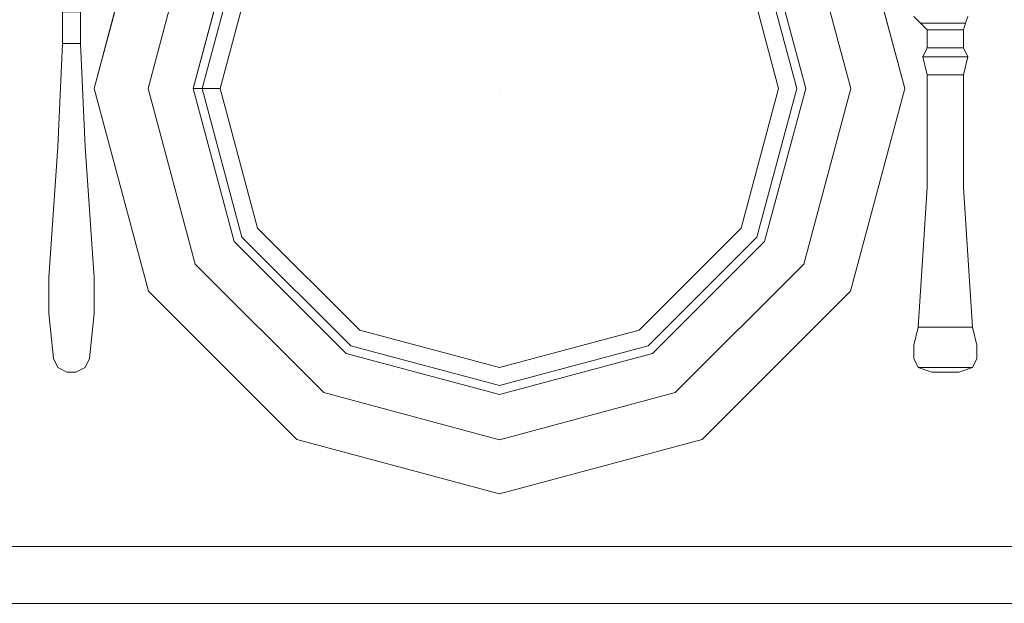
# Model space of a CAD drawing. Units: inches. Extents: x 375 to 1122, y 27 to 1069.
# Tile 10 of 155: x 719.12 to 732.58, y 254.7 to 262.68. Entities that reach past the tile are written whole.
import ezdxf

# ---------------------------------------------------------------- set-up
doc = ezdxf.new("R2010")
doc.units = ezdxf.units.IN
doc.layers.add('Furniture', color=30, linetype='Continuous', lineweight=18)

# ---------------------------------------------------------------- blocks, each defined once
blk = doc.blocks.new('A$C403C54AD')
for p, q in [((2.27071, 1.26108, -0.0006), (2.27071, 0.79569, -0.0006)), ((2.2901, 1.26108, -0.0006), (2.2901, 0.79569, -0.0006))]:
    blk.add_line(p, q)
for points, invisible_edges in [([(2.19569, 1.17996, -0.05014), (2.19569, 1.16149, -0.05014), (2.20185, 1.15995, -0.0486), (2.20185, 1.1815, -0.0486)], 4), ([(2.19569, 1.17996, -0.05938), (2.19569, 1.16149, -0.05938), (2.20185, 1.15995, -0.06091), (2.20185, 1.1815, -0.06091)], 4), ([(2.20185, 1.15995, -0.0486), (2.20185, 1.1815, -0.0486), (2.20647, 1.1815, -0.05014), (2.20647, 1.15995, -0.05014)], 5), ([(2.20185, 1.15995, -0.06091), (2.20185, 1.1815, -0.06091), (2.20647, 1.1815, -0.05938), (2.20647, 1.15995, -0.05938)], 5), ([(2.20647, 1.1815, -0.05014), (2.20647, 1.15995, -0.05014), (2.20954, 1.16149, -0.05168), (2.20954, 1.17996, -0.05168)], 1), ([(2.20647, 1.1815, -0.05938), (2.20647, 1.15995, -0.05938), (2.20954, 1.16149, -0.05784), (2.20954, 1.17996, -0.05784)], 1), ([(2.08949, 1.15995, -0.05399), (2.08949, 1.17842, -0.05399), (2.0918, 1.17765, -0.05322), (2.0918, 1.16226, -0.05322)], 1), ([(2.08949, 1.15995, -0.05553), (2.08949, 1.17842, -0.05553), (2.0918, 1.17765, -0.0563), (2.0918, 1.16226, -0.0563)], 1), ([(2.0918, 1.17765, -0.0563), (2.0918, 1.17765, -0.05322), (2.08949, 1.17842, -0.05399), (2.08949, 1.17842, -0.05553)], 5), ([(2.0941, 1.17688, -0.05014), (2.0941, 1.17688, -0.05938), (2.0918, 1.17765, -0.0563), (2.0918, 1.17765, -0.05322)], 5), ([(2.14798, 1.17688, -0.0486), (2.14798, 1.16457, -0.0486), (2.17106, 1.16303, -0.0486), (2.17106, 1.17842, -0.0486)], 5), ([(2.14798, 1.17688, -0.06091), (2.14798, 1.16457, -0.06091), (2.17106, 1.16303, -0.06091), (2.17106, 1.17842, -0.06091)], 5), ([(2.17106, 1.16303, -0.0486), (2.17106, 1.17842, -0.0486), (2.19569, 1.17996, -0.05014), (2.19569, 1.16149, -0.05014)], 1), ([(2.17106, 1.16303, -0.06091), (2.17106, 1.17842, -0.06091), (2.19569, 1.17996, -0.05938), (2.19569, 1.16149, -0.05938)], 1), ([(2.10026, 1.17688, -0.05938), (2.10026, 1.17688, -0.05014), (2.0941, 1.17688, -0.05014), (2.0941, 1.17688, -0.05938)], 4), ([(2.1095, 1.16457, -0.05014), (2.1095, 1.17688, -0.05014), (2.14798, 1.17688, -0.0486), (2.14798, 1.16457, -0.0486)], 4), ([(2.1095, 1.16457, -0.05938), (2.1095, 1.17688, -0.05938), (2.14798, 1.17688, -0.06091), (2.14798, 1.16457, -0.06091)], 4), ([(2.0918, 1.16226, -0.05322), (2.0918, 1.16226, -0.0563), (2.0941, 1.16457, -0.05938), (2.0941, 1.16457, -0.05014)], 5), ([(2.0941, 1.16457, -0.05938), (2.0941, 1.16457, -0.05014), (2.10026, 1.16457, -0.05014), (2.10026, 1.16457, -0.05938)], 1), ([(2.08949, 1.15995, -0.05553), (2.08949, 1.15995, -0.05399), (2.0918, 1.16226, -0.05322), (2.0918, 1.16226, -0.0563)], 5), ([(2.17876, 0.86443, -0.04825), (2.17876, 0.87982, -0.04825), (2.13412, 0.87674, -0.04587), (2.13412, 0.8675, -0.04587)], 5), ([(2.17876, 0.86443, -0.05289), (2.17876, 0.87982, -0.05289), (2.13412, 0.87674, -0.04895), (2.13412, 0.8675, -0.04895)], 5), ([(2.17876, 0.87982, -0.05289), (2.17876, 0.87982, -0.04825), (2.13412, 0.87674, -0.04587), (2.13412, 0.87674, -0.04895)], 4), ([(2.19107, 0.87982, -0.04858), (2.19107, 0.86443, -0.04858), (2.17876, 0.86443, -0.04825), (2.17876, 0.87982, -0.04825)], 5), ([(2.19107, 0.87982, -0.05321), (2.19107, 0.86443, -0.05321), (2.17876, 0.86443, -0.05289), (2.17876, 0.87982, -0.05289)], 5), ([(2.20647, 0.86596, -0.04855), (2.20647, 0.87828, -0.04855), (2.19107, 0.87982, -0.04858), (2.19107, 0.86443, -0.04858)], 5), ([(2.20647, 0.86596, -0.05318), (2.20647, 0.87828, -0.05318), (2.19107, 0.87982, -0.05321), (2.19107, 0.86443, -0.05321)], 5), ([(2.20954, 0.87674, -0.0483), (2.20954, 0.8675, -0.0483), (2.20647, 0.86596, -0.04855), (2.20647, 0.87828, -0.04855)], 5), ([(2.20954, 0.87674, -0.05294), (2.20954, 0.8675, -0.05294), (2.20647, 0.86596, -0.05318), (2.20647, 0.87828, -0.05318)], 5), ([(2.09872, 0.8752, -0.04555), (2.09872, 0.8752, -0.04296), (2.08795, 0.8752, -0.04504), (2.08795, 0.8752, -0.04763)], 5), ([(2.13412, 0.87674, -0.04587), (2.13412, 0.8675, -0.04587), (2.09872, 0.86904, -0.04296), (2.09872, 0.8752, -0.04296)], 1), ([(2.13412, 0.87674, -0.04587), (2.13412, 0.87674, -0.04895), (2.09872, 0.8752, -0.04555), (2.09872, 0.8752, -0.04296)], 5), ([(2.13412, 0.87674, -0.04895), (2.13412, 0.8675, -0.04895), (2.09872, 0.86904, -0.04555), (2.09872, 0.8752, -0.04555)], 1), ([(2.21108, 0.87058, -0.04847), (2.21108, 0.87366, -0.04847), (2.20954, 0.87674, -0.0483), (2.20954, 0.8675, -0.0483)], 4), ([(2.21108, 0.87058, -0.0526), (2.21108, 0.87366, -0.0526), (2.20954, 0.87674, -0.05294), (2.20954, 0.8675, -0.05294)], 4), ([(2.08795, 0.86904, -0.04763), (2.08795, 0.86904, -0.04504), (2.09872, 0.86904, -0.04296), (2.09872, 0.86904, -0.04555)], 5), ([(2.09872, 0.86904, -0.04296), (2.09872, 0.86904, -0.04555), (2.13412, 0.8675, -0.04895), (2.13412, 0.8675, -0.04587)], 5), ([(2.13412, 0.8675, -0.04895), (2.13412, 0.8675, -0.04587), (2.17876, 0.86443, -0.04825), (2.17876, 0.86443, -0.05289)], 1)]:
    blk.add_3dface(points, dxfattribs=dict(invisible_edges=invisible_edges))
for points in [[(2.20185, 1.1815, -0.06091), (2.20185, 1.1815, -0.0486), (2.19569, 1.17996, -0.05014), (2.19569, 1.17996, -0.05938)], [(2.20647, 1.1815, -0.05014), (2.20647, 1.1815, -0.05938), (2.20185, 1.1815, -0.06091), (2.20185, 1.1815, -0.0486)], [(2.20954, 1.17996, -0.05168), (2.20954, 1.17996, -0.05784), (2.20647, 1.1815, -0.05938), (2.20647, 1.1815, -0.05014)], [(2.0918, 1.16226, -0.05322), (2.0918, 1.17765, -0.05322), (2.0941, 1.17688, -0.05014), (2.0941, 1.16457, -0.05014)], [(2.0918, 1.16226, -0.0563), (2.0918, 1.17765, -0.0563), (2.0941, 1.17688, -0.05938), (2.0941, 1.16457, -0.05938)], [(2.10026, 1.16457, -0.05014), (2.10026, 1.17688, -0.05014), (2.10334, 1.17842, -0.0486), (2.10334, 1.16303, -0.0486)], [(2.10026, 1.16457, -0.05938), (2.10026, 1.17688, -0.05938), (2.10334, 1.17842, -0.06091), (2.10334, 1.16303, -0.06091)], [(2.10334, 1.17842, -0.0486), (2.10334, 1.17842, -0.06091), (2.10026, 1.17688, -0.05938), (2.10026, 1.17688, -0.05014)], [(2.10334, 1.17842, -0.0486), (2.10334, 1.16303, -0.0486), (2.1095, 1.16457, -0.05014), (2.1095, 1.17688, -0.05014)], [(2.10334, 1.17842, -0.06091), (2.10334, 1.16303, -0.06091), (2.1095, 1.16457, -0.05938), (2.1095, 1.17688, -0.05938)], [(2.1095, 1.17688, -0.05938), (2.1095, 1.17688, -0.05014), (2.10334, 1.17842, -0.0486), (2.10334, 1.17842, -0.06091)], [(2.17106, 1.17842, -0.06091), (2.17106, 1.17842, -0.0486), (2.14798, 1.17688, -0.0486), (2.14798, 1.17688, -0.06091)], [(2.19569, 1.17996, -0.05014), (2.19569, 1.17996, -0.05938), (2.17106, 1.17842, -0.06091), (2.17106, 1.17842, -0.0486)], [(2.20954, 1.16149, -0.05168), (2.20954, 1.17996, -0.05168), (2.21108, 1.17534, -0.05476), (2.21108, 1.16611, -0.05476)], [(2.21108, 1.17534, -0.05476), (2.21108, 1.17534, -0.05476), (2.20954, 1.17996, -0.05168), (2.20954, 1.17996, -0.05784)], [(2.20954, 1.16149, -0.05784), (2.20954, 1.17996, -0.05784), (2.21108, 1.17534, -0.05476), (2.21108, 1.16611, -0.05476)], [(2.0941, 1.17688, -0.05014), (2.0941, 1.16457, -0.05014), (2.10026, 1.16457, -0.05014), (2.10026, 1.17688, -0.05014)], [(2.0941, 1.17688, -0.05938), (2.0941, 1.16457, -0.05938), (2.10026, 1.16457, -0.05938), (2.10026, 1.17688, -0.05938)], [(2.14798, 1.17688, -0.0486), (2.14798, 1.17688, -0.06091), (2.1095, 1.17688, -0.05938), (2.1095, 1.17688, -0.05014)], [(2.10026, 1.16457, -0.05014), (2.10026, 1.16457, -0.05938), (2.10334, 1.16303, -0.06091), (2.10334, 1.16303, -0.0486)], [(2.10334, 1.16303, -0.06091), (2.10334, 1.16303, -0.0486), (2.1095, 1.16457, -0.05014), (2.1095, 1.16457, -0.05938)], [(2.1095, 1.16457, -0.05014), (2.1095, 1.16457, -0.05938), (2.14798, 1.16457, -0.06091), (2.14798, 1.16457, -0.0486)], [(2.14798, 1.16457, -0.06091), (2.14798, 1.16457, -0.0486), (2.17106, 1.16303, -0.0486), (2.17106, 1.16303, -0.06091)], [(2.20954, 1.16149, -0.05168), (2.20954, 1.16149, -0.05784), (2.21108, 1.16611, -0.05476)], [(2.17106, 1.16303, -0.0486), (2.17106, 1.16303, -0.06091), (2.19569, 1.16149, -0.05938), (2.19569, 1.16149, -0.05014)], [(2.19569, 1.16149, -0.05938), (2.19569, 1.16149, -0.05014), (2.20185, 1.15995, -0.0486), (2.20185, 1.15995, -0.06091)], [(2.20647, 1.15995, -0.05938), (2.20647, 1.15995, -0.05014), (2.20954, 1.16149, -0.05168), (2.20954, 1.16149, -0.05784)], [(2.20185, 1.15995, -0.0486), (2.20185, 1.15995, -0.06091), (2.20647, 1.15995, -0.05938), (2.20647, 1.15995, -0.05014)], [(2.19107, 0.87982, -0.04858), (2.19107, 0.87982, -0.05321), (2.17876, 0.87982, -0.05289), (2.17876, 0.87982, -0.04825)], [(2.20647, 0.87828, -0.05318), (2.20647, 0.87828, -0.04855), (2.19107, 0.87982, -0.04858), (2.19107, 0.87982, -0.05321)], [(2.20954, 0.87674, -0.0483), (2.20954, 0.87674, -0.05294), (2.20647, 0.87828, -0.05318), (2.20647, 0.87828, -0.04855)], [(2.09872, 0.86904, -0.04296), (2.09872, 0.8752, -0.04296), (2.08795, 0.8752, -0.04504), (2.08795, 0.86904, -0.04504)], [(2.09872, 0.86904, -0.04555), (2.09872, 0.8752, -0.04555), (2.08795, 0.8752, -0.04763), (2.08795, 0.86904, -0.04763)], [(2.21108, 0.87366, -0.0526), (2.21108, 0.87366, -0.04847), (2.20954, 0.87674, -0.0483), (2.20954, 0.87674, -0.05294)], [(2.21108, 0.87058, -0.04847), (2.21108, 0.87058, -0.0526), (2.21108, 0.87366, -0.0526), (2.21108, 0.87366, -0.04847)], [(2.20954, 0.8675, -0.05294), (2.20954, 0.8675, -0.0483), (2.21108, 0.87058, -0.04847), (2.21108, 0.87058, -0.0526)], [(2.19107, 0.86443, -0.05321), (2.19107, 0.86443, -0.04858), (2.20647, 0.86596, -0.04855), (2.20647, 0.86596, -0.05318)], [(2.20647, 0.86596, -0.04855), (2.20647, 0.86596, -0.05318), (2.20954, 0.8675, -0.05294), (2.20954, 0.8675, -0.0483)], [(2.17876, 0.86443, -0.04825), (2.17876, 0.86443, -0.05289), (2.19107, 0.86443, -0.05321), (2.19107, 0.86443, -0.04858)]]:
    blk.add_3dface(points)
at = {"linetype": 'ByBlock'}
for points, invisible_edges in [([(2.11411, 1.15687, -0.03783), (2.11411, 1.1384, -0.03783), (2.05409, 1.12232, -0.03783), (2.04485, 1.13831, -0.03783)], 5), ([(2.11411, 1.12301, -0.05168), (2.11411, 1.15687, -0.04244), (2.04485, 1.13831, -0.04244), (2.06178, 1.10899, -0.05168)], 5), ([(2.18338, 1.13831, -0.03783), (2.17414, 1.12232, -0.03783), (2.11411, 1.1384, -0.03783), (2.11411, 1.15687, -0.03783)], 5), ([(2.16645, 1.10899, -0.05168), (2.18338, 1.13831, -0.04244), (2.11411, 1.15687, -0.04244), (2.11411, 1.12301, -0.05168)], 5), ([(2.11411, 1.1384, -0.03783), (2.11411, 1.11993, -0.04398), (2.06332, 1.10632, -0.04398), (2.05409, 1.12232, -0.03783)], 5), ([(2.17414, 1.12232, -0.03783), (2.16491, 1.10632, -0.04398), (2.11411, 1.11993, -0.04398), (2.11411, 1.1384, -0.03783)], 5), ([(2.20476, 1.07068, -0.05168), (2.23408, 1.08761, -0.04244), (2.18338, 1.13831, -0.04244), (2.16645, 1.10899, -0.05168)], 5), ([(2.23408, 1.08761, -0.03783), (2.21809, 1.07837, -0.03783), (2.17414, 1.12232, -0.03783), (2.18338, 1.13831, -0.03783)], 5), ([(2.11411, 1.11377, -0.06091), (2.11411, 1.12301, -0.05168), (2.06178, 1.10899, -0.05168), (2.0664, 1.10099, -0.06091)], 5), ([(2.16183, 1.10099, -0.06091), (2.16645, 1.10899, -0.05168), (2.11411, 1.12301, -0.05168), (2.11411, 1.11377, -0.06091)], 5), ([(2.21809, 1.07837, -0.03783), (2.20209, 1.06914, -0.04398), (2.16491, 1.10632, -0.04398), (2.17414, 1.12232, -0.03783)], 5), ([(2.11411, 1.11993, -0.04398), (2.11411, 1.01834, -0.04398), (2.11411, 1.01834, -0.04398), (2.06332, 1.10632, -0.04398)], 5), ([(2.16491, 1.10632, -0.04398), (2.11411, 1.01834, -0.04398), (2.11411, 1.01834, -0.04398), (2.11411, 1.11993, -0.04398)], 5), ([(2.19676, 1.06606, -0.06091), (2.20476, 1.07068, -0.05168), (2.16645, 1.10899, -0.05168), (2.16183, 1.10099, -0.06091)], 5), ([(2.06332, 1.10632, -0.04398), (2.11411, 1.01834, -0.04398), (2.11411, 1.01834, -0.04398), (2.02614, 1.06914, -0.04398)], 5), ([(2.20209, 1.06914, -0.04398), (2.11411, 1.01834, -0.04398), (2.11411, 1.01834, -0.04398), (2.16491, 1.10632, -0.04398)], 5), ([(2.21878, 1.01834, -0.05168), (2.25264, 1.01834, -0.04244), (2.23408, 1.08761, -0.04244), (2.20476, 1.07068, -0.05168)], 5), ([(2.25264, 1.01834, -0.03783), (2.23417, 1.01834, -0.03783), (2.21809, 1.07837, -0.03783), (2.23408, 1.08761, -0.03783)], 5), ([(2.23417, 1.01834, -0.03783), (2.2157, 1.01834, -0.04398), (2.20209, 1.06914, -0.04398), (2.21809, 1.07837, -0.03783)], 5), ([(2.20954, 1.01834, -0.06091), (2.21878, 1.01834, -0.05168), (2.20476, 1.07068, -0.05168), (2.19676, 1.06606, -0.06091)], 5), ([(2.02614, 1.06914, -0.04398), (2.11411, 1.01834, -0.04398), (2.11411, 1.01834, -0.04398), (2.01253, 1.01834, -0.04398)], 5), ([(2.2157, 1.01834, -0.04398), (2.11411, 1.01834, -0.04398), (2.11411, 1.01834, -0.04398), (2.20209, 1.06914, -0.04398)], 5), ([(2.01253, 1.01834, -0.04398), (2.11411, 1.01834, -0.04398), (2.11411, 1.01834, -0.04398), (2.02614, 0.96755, -0.04398)], 5), ([(2.02614, 0.96755, -0.04398), (2.11411, 1.01834, -0.04398), (2.11411, 1.01834, -0.04398), (2.06332, 0.93037, -0.04398)], 5), ([(2.06332, 0.93037, -0.04398), (2.11411, 1.01834, -0.04398), (2.11411, 1.01834, -0.04398), (2.11411, 0.91676, -0.04398)], 5), ([(2.20209, 0.96755, -0.04398), (2.11411, 1.01834, -0.04398), (2.11411, 1.01834, -0.04398), (2.2157, 1.01834, -0.04398)], 5), ([(2.16491, 0.93037, -0.04398), (2.11411, 1.01834, -0.04398), (2.11411, 1.01834, -0.04398), (2.20209, 0.96755, -0.04398)], 5), ([(2.11411, 0.91676, -0.04398), (2.11411, 1.01834, -0.04398), (2.11411, 1.01834, -0.04398), (2.16491, 0.93037, -0.04398)], 5), ([(2.19676, 0.97063, -0.06091), (2.20476, 0.96601, -0.05168), (2.21878, 1.01834, -0.05168), (2.20954, 1.01834, -0.06091)], 5), ([(2.21809, 0.95832, -0.03783), (2.20209, 0.96755, -0.04398), (2.2157, 1.01834, -0.04398), (2.23417, 1.01834, -0.03783)], 5), ([(2.20476, 0.96601, -0.05168), (2.23408, 0.94908, -0.04244), (2.25264, 1.01834, -0.04244), (2.21878, 1.01834, -0.05168)], 5), ([(2.23408, 0.94908, -0.03783), (2.21809, 0.95832, -0.03783), (2.23417, 1.01834, -0.03783), (2.25264, 1.01834, -0.03783)], 5), ([(2.16183, 0.9357, -0.06091), (2.16645, 0.9277, -0.05168), (2.20476, 0.96601, -0.05168), (2.19676, 0.97063, -0.06091)], 5), ([(2.17414, 0.91437, -0.03783), (2.16491, 0.93037, -0.04398), (2.20209, 0.96755, -0.04398), (2.21809, 0.95832, -0.03783)], 5), ([(2.16645, 0.9277, -0.05168), (2.18338, 0.89838, -0.04244), (2.23408, 0.94908, -0.04244), (2.20476, 0.96601, -0.05168)], 5), ([(2.18338, 0.89838, -0.03783), (2.17414, 0.91437, -0.03783), (2.21809, 0.95832, -0.03783), (2.23408, 0.94908, -0.03783)], 5), ([(2.11411, 0.92291, -0.06091), (2.11411, 0.91368, -0.05168), (2.16645, 0.9277, -0.05168), (2.16183, 0.9357, -0.06091)], 4), ([(2.05409, 0.91437, -0.03783), (2.06332, 0.93037, -0.04398), (2.11411, 0.91676, -0.04398), (2.11411, 0.89829, -0.03783)], 5), ([(2.11411, 0.89829, -0.03783), (2.11411, 0.91676, -0.04398), (2.16491, 0.93037, -0.04398), (2.17414, 0.91437, -0.03783)], 5), ([(2.06178, 0.9277, -0.05168), (2.04485, 0.89838, -0.04244), (2.11411, 0.87982, -0.04244), (2.11411, 0.91368, -0.05168)], 5), ([(2.11411, 0.91368, -0.05168), (2.11411, 0.87982, -0.04244), (2.18338, 0.89838, -0.04244), (2.16645, 0.9277, -0.05168)], 5), ([(2.04485, 0.89838, -0.03783), (2.05409, 0.91437, -0.03783), (2.11411, 0.89829, -0.03783), (2.11411, 0.87982, -0.03783)], 5), ([(2.11411, 0.87982, -0.03783), (2.11411, 0.89829, -0.03783), (2.17414, 0.91437, -0.03783), (2.18338, 0.89838, -0.03783)], 5)]:
    blk.add_3dface(points, dxfattribs=dict(at, invisible_edges=invisible_edges))
for points in [[(2.11411, 1.15687, -0.04244), (2.11411, 1.15687, -0.03783), (2.04485, 1.13831, -0.03783), (2.04485, 1.13831, -0.04244)], [(2.18338, 1.13831, -0.04244), (2.18338, 1.13831, -0.03783), (2.11411, 1.15687, -0.03783), (2.11411, 1.15687, -0.04244)], [(2.23408, 1.08761, -0.04244), (2.23408, 1.08761, -0.03783), (2.18338, 1.13831, -0.03783), (2.18338, 1.13831, -0.04244)], [(2.25264, 1.01834, -0.04244), (2.25264, 1.01834, -0.03783), (2.23408, 1.08761, -0.03783), (2.23408, 1.08761, -0.04244)], [(2.23408, 0.94908, -0.04244), (2.23408, 0.94908, -0.03783), (2.25264, 1.01834, -0.03783), (2.25264, 1.01834, -0.04244)], [(2.18338, 0.89838, -0.04244), (2.18338, 0.89838, -0.03783), (2.23408, 0.94908, -0.03783), (2.23408, 0.94908, -0.04244)], [(2.0664, 0.9357, -0.06091), (2.06178, 0.9277, -0.05168), (2.11411, 0.91368, -0.05168), (2.11411, 0.92291, -0.06091)], [(2.04485, 0.89838, -0.04244), (2.04485, 0.89838, -0.03783), (2.11411, 0.87982, -0.03783), (2.11411, 0.87982, -0.04244)], [(2.11411, 0.87982, -0.04244), (2.11411, 0.87982, -0.03783), (2.18338, 0.89838, -0.03783), (2.18338, 0.89838, -0.04244)]]:
    blk.add_3dface(points, dxfattribs=at)

msp = doc.modelspace()

# ---------------------------------------------------------------- block references
at = {"layer": 'Furniture', "xscale": 39.9918517141215, "yscale": 39.9918517141215, "zscale": 39.9918517141215, "rotation": 270}
msp.add_blockref('A$C403C54AD', (684.955, 346.287, 0.024), dxfattribs=at)

doc.saveas('drawing.dxf')
